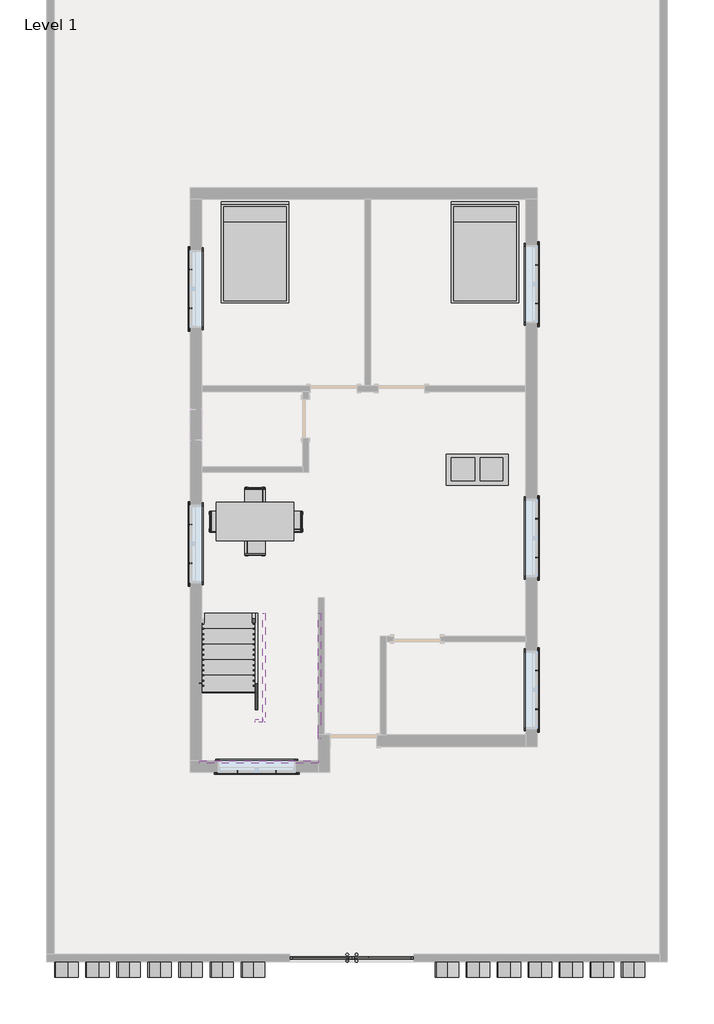
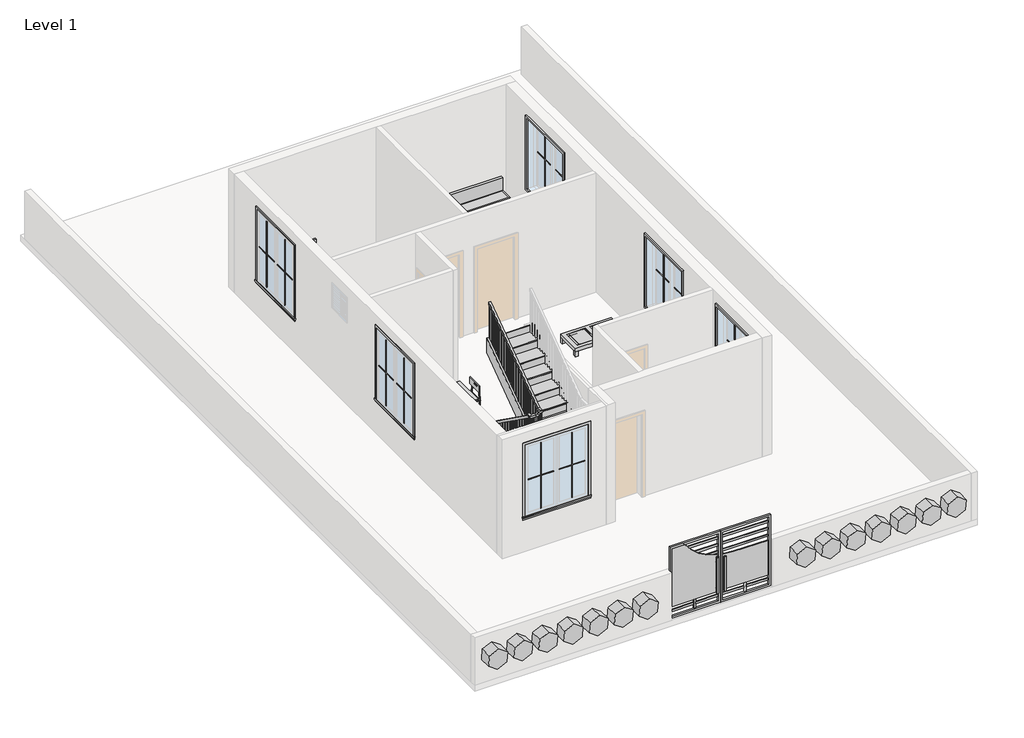
# One storey, part 3 of 3: 40 proxies, 6 members, 3 furniture elements, 1 railing, 1 stair flight.
"""IFC4 building model written with IfcOpenShell, lengths in millimetres."""

from ifc_helpers import new_model, si_unit, frame, origin, place, context, project, spatial, polyline, outline, extrude, faceted_brep, transform, mapped, element, save
from components import generic_models_113f6068, generic_models_1_generic_models_1_1536aad0, generic_models_10_generic_models_1_a884c7fe, generic_models_11_generic_models_1_35dd710a, generic_models_12_generic_models_1_297bb3a6, generic_models_13_generic_models_1_cefb3180, generic_models_14_generic_models_1_e19c2567, generic_models_2_generic_models_1_b64329ca, generic_models_3_generic_models_1_4242ebdf, generic_models_4_generic_models_1_f88cb9c1, generic_models_5_generic_models_1_6c1de215, generic_models_6_generic_models_1_f976f914, generic_models_7_generic_models_1_dc570d8e, generic_models_8_generic_models_1_e8626bb7, generic_models_9_generic_models_1_6881e9d4, muntin_pattern_2x2_muntin_pattern_2x2_f6a80940, muntin_pattern_2x2_muntin_pattern_2x2_09b00a1c, trim_window_exterior_flat_with_sill_698ed857, trim_window_interior_flat_picture_frame_92551a5e, coffee_table_with_brass_mullions_11320_coffee_table_with_5962bef7, bed_17739_bed_17739_15c61121, dining_table_w_chairs_11374_0cdfc61b, stair_flight_d468406d

model = new_model("IFC4")

# Units and contexts
model_context = context("Model", 3, world=origin())
ifc_project = project(units=[si_unit("LENGTHUNIT", "METRE", prefix="MILLI")], contexts=[model_context])

# Site, building, storey
site = spatial("IfcSite", under=ifc_project)
building = spatial("IfcBuilding", under=site)
storey = spatial("IfcBuildingStorey", under=building, Name="Level 1", Elevation=0.0)

# Proxies
placement = place(None, origin())
generic_models_shape = generic_models_113f6068(model_context)
element("IfcBuildingElementProxy", 1, Name="Generic Models", at=placement, inside=storey, context=model_context, shape_type="MappedRepresentation", body=[
    mapped(generic_models_shape, transform((-1286.5514601, -10313.9372434, 0.0), x_axis=(1.0, 0.0, 0.0), y_axis=(0.0, 1.0, 0.0), z_axis=(0.0, 0.0, 1.0))),
])
generic_models_1_generic_models_1_shape = generic_models_1_generic_models_1_1536aad0(model_context)
element("IfcBuildingElementProxy", 2, Name="Generic Models 1 : Generic Models 1", ObjectType="Generic Models 1 : Generic Models 1", at=placement, inside=storey, context=model_context, shape_type="MappedRepresentation", body=[
    mapped(generic_models_1_generic_models_1_shape, transform((0.0, 0.0, 0.0), x_axis=(1.0, 0.0, 0.0), y_axis=(0.0, 1.0, 0.0), z_axis=(0.0, 0.0, 1.0))),
])
generic_models_10_generic_models_1_shape = generic_models_10_generic_models_1_a884c7fe(model_context)
element("IfcBuildingElementProxy", 3, Name="Generic Models 10 : Generic Models 1", ObjectType="Generic Models 10 : Generic Models 1", at=placement, inside=storey, context=model_context, shape_type="MappedRepresentation", body=[
    mapped(generic_models_10_generic_models_1_shape, transform((0.0, 0.0, 0.0), x_axis=(1.0, 0.0, 0.0), y_axis=(0.0, 1.0, 0.0), z_axis=(0.0, 0.0, 1.0))),
])
generic_models_11_generic_models_1_shape = generic_models_11_generic_models_1_35dd710a(model_context)
element("IfcBuildingElementProxy", 4, Name="Generic Models 11 : Generic Models 1", ObjectType="Generic Models 11 : Generic Models 1", at=placement, inside=storey, context=model_context, shape_type="MappedRepresentation", body=[
    mapped(generic_models_11_generic_models_1_shape, transform((0.0, 0.0, 0.0), x_axis=(1.0, 0.0, 0.0), y_axis=(0.0, 1.0, 0.0), z_axis=(0.0, 0.0, 1.0))),
])
generic_models_12_generic_models_1_shape = generic_models_12_generic_models_1_297bb3a6(model_context)
element("IfcBuildingElementProxy", 5, Name="Generic Models 12 : Generic Models 1", ObjectType="Generic Models 12 : Generic Models 1", at=placement, inside=storey, context=model_context, shape_type="MappedRepresentation", body=[
    mapped(generic_models_12_generic_models_1_shape, transform((0.0, 0.0, 0.0), x_axis=(1.0, 0.0, 0.0), y_axis=(0.0, 1.0, 0.0), z_axis=(0.0, 0.0, 1.0))),
])
generic_models_13_generic_models_1_shape = generic_models_13_generic_models_1_cefb3180(model_context)
element("IfcBuildingElementProxy", 6, Name="Generic Models 13 : Generic Models 1", ObjectType="Generic Models 13 : Generic Models 1", at=placement, inside=storey, context=model_context, shape_type="MappedRepresentation", body=[
    mapped(generic_models_13_generic_models_1_shape, transform((0.0, 0.0, 0.0), x_axis=(1.0, 0.0, 0.0), y_axis=(0.0, 1.0, 0.0), z_axis=(0.0, 0.0, 1.0))),
])
generic_models_14_generic_models_1_shape = generic_models_14_generic_models_1_e19c2567(model_context)
element("IfcBuildingElementProxy", 7, Name="Generic Models 14 : Generic Models 1", ObjectType="Generic Models 14 : Generic Models 1", at=placement, inside=storey, context=model_context, shape_type="MappedRepresentation", body=[
    mapped(generic_models_14_generic_models_1_shape, transform((0.0, 0.0, 0.0), x_axis=(1.0, 0.0, 0.0), y_axis=(0.0, 1.0, 0.0), z_axis=(0.0, 0.0, 1.0))),
])
generic_models_2_generic_models_1_shape = generic_models_2_generic_models_1_b64329ca(model_context)
element("IfcBuildingElementProxy", 8, Name="Generic Models 2 : Generic Models 1", ObjectType="Generic Models 2 : Generic Models 1", at=placement, inside=storey, context=model_context, shape_type="MappedRepresentation", body=[
    mapped(generic_models_2_generic_models_1_shape, transform((0.0, 0.0, 0.0), x_axis=(1.0, 0.0, 0.0), y_axis=(0.0, 1.0, 0.0), z_axis=(0.0, 0.0, 1.0))),
])
generic_models_3_generic_models_1_shape = generic_models_3_generic_models_1_4242ebdf(model_context)
element("IfcBuildingElementProxy", 9, Name="Generic Models 3 : Generic Models 1", ObjectType="Generic Models 3 : Generic Models 1", at=placement, inside=storey, context=model_context, shape_type="MappedRepresentation", body=[
    mapped(generic_models_3_generic_models_1_shape, transform((0.0, 0.0, 0.0), x_axis=(1.0, 0.0, 0.0), y_axis=(0.0, 1.0, 0.0), z_axis=(0.0, 0.0, 1.0))),
])
generic_models_4_generic_models_1_shape = generic_models_4_generic_models_1_f88cb9c1(model_context)
element("IfcBuildingElementProxy", 10, Name="Generic Models 4 : Generic Models 1", ObjectType="Generic Models 4 : Generic Models 1", at=placement, inside=storey, context=model_context, shape_type="MappedRepresentation", body=[
    mapped(generic_models_4_generic_models_1_shape, transform((0.0, 0.0, 0.0), x_axis=(1.0, 0.0, 0.0), y_axis=(0.0, 1.0, 0.0), z_axis=(0.0, 0.0, 1.0))),
])
generic_models_5_generic_models_1_shape = generic_models_5_generic_models_1_6c1de215(model_context)
element("IfcBuildingElementProxy", 11, Name="Generic Models 5 : Generic Models 1", ObjectType="Generic Models 5 : Generic Models 1", at=placement, inside=storey, context=model_context, shape_type="MappedRepresentation", body=[
    mapped(generic_models_5_generic_models_1_shape, transform((0.0, 0.0, 0.0), x_axis=(1.0, 0.0, 0.0), y_axis=(0.0, 1.0, 0.0), z_axis=(0.0, 0.0, 1.0))),
])
generic_models_6_generic_models_1_shape = generic_models_6_generic_models_1_f976f914(model_context)
element("IfcBuildingElementProxy", 12, Name="Generic Models 6 : Generic Models 1", ObjectType="Generic Models 6 : Generic Models 1", at=placement, inside=storey, context=model_context, shape_type="MappedRepresentation", body=[
    mapped(generic_models_6_generic_models_1_shape, transform((0.0, 0.0, 0.0), x_axis=(1.0, 0.0, 0.0), y_axis=(0.0, 1.0, 0.0), z_axis=(0.0, 0.0, 1.0))),
])
generic_models_7_generic_models_1_shape = generic_models_7_generic_models_1_dc570d8e(model_context)
element("IfcBuildingElementProxy", 13, Name="Generic Models 7 : Generic Models 1", ObjectType="Generic Models 7 : Generic Models 1", at=placement, inside=storey, context=model_context, shape_type="MappedRepresentation", body=[
    mapped(generic_models_7_generic_models_1_shape, transform((0.0, 0.0, 0.0), x_axis=(1.0, 0.0, 0.0), y_axis=(0.0, 1.0, 0.0), z_axis=(0.0, 0.0, 1.0))),
])
generic_models_8_generic_models_1_shape = generic_models_8_generic_models_1_e8626bb7(model_context)
element("IfcBuildingElementProxy", 14, Name="Generic Models 8 : Generic Models 1", ObjectType="Generic Models 8 : Generic Models 1", at=placement, inside=storey, context=model_context, shape_type="MappedRepresentation", body=[
    mapped(generic_models_8_generic_models_1_shape, transform((0.0, 0.0, 0.0), x_axis=(1.0, 0.0, 0.0), y_axis=(0.0, 1.0, 0.0), z_axis=(0.0, 0.0, 1.0))),
])
generic_models_9_generic_models_1_shape = generic_models_9_generic_models_1_6881e9d4(model_context)
element("IfcBuildingElementProxy", 15, Name="Generic Models 9 : Generic Models 1", ObjectType="Generic Models 9 : Generic Models 1", at=placement, inside=storey, context=model_context, shape_type="MappedRepresentation", body=[
    mapped(generic_models_9_generic_models_1_shape, transform((0.0, 0.0, 0.0), x_axis=(1.0, 0.0, 0.0), y_axis=(0.0, 1.0, 0.0), z_axis=(0.0, 0.0, 1.0))),
])
muntin_pattern_2x2_muntin_pattern_2x2_shape = muntin_pattern_2x2_muntin_pattern_2x2_f6a80940(model_context)
element("IfcBuildingElementProxy", 16, Name="Muntin Pattern_2x2 : Muntin Pattern_2x2", ObjectType="Muntin Pattern_2x2 : Muntin Pattern_2x2", at=placement, inside=storey, context=model_context, shape_type="MappedRepresentation", body=[
    mapped(muntin_pattern_2x2_muntin_pattern_2x2_shape, transform((-2773.368364, -6686.2830018, 984.25), x_axis=(-1.0, 0.0, 0.0), y_axis=(0.0, -1.0, 0.0), z_axis=(0.0, 0.0, 1.0))),
])
element("IfcBuildingElementProxy", 17, Name="Muntin Pattern_2x2 : Muntin Pattern_2x2", ObjectType="Muntin Pattern_2x2 : Muntin Pattern_2x2", at=placement, inside=storey, context=model_context, shape_type="MappedRepresentation", body=[
    mapped(muntin_pattern_2x2_muntin_pattern_2x2_shape, transform((2349.494136, -4693.9705018, 984.25), x_axis=(0.0, -1.0, 0.0), y_axis=(1.0, 0.0, 0.0), z_axis=(0.0, 0.0, 1.0))),
])
element("IfcBuildingElementProxy", 18, Name="Muntin Pattern_2x2 : Muntin Pattern_2x2", ObjectType="Muntin Pattern_2x2 : Muntin Pattern_2x2", at=placement, inside=storey, context=model_context, shape_type="MappedRepresentation", body=[
    mapped(muntin_pattern_2x2_muntin_pattern_2x2_shape, transform((2349.494136, -1712.6455018, 984.25), x_axis=(0.0, -1.0, 0.0), y_axis=(1.0, 0.0, 0.0), z_axis=(0.0, 0.0, 1.0))),
])
element("IfcBuildingElementProxy", 19, Name="Muntin Pattern_2x2 : Muntin Pattern_2x2", ObjectType="Muntin Pattern_2x2 : Muntin Pattern_2x2", at=placement, inside=storey, context=model_context, shape_type="MappedRepresentation", body=[
    mapped(muntin_pattern_2x2_muntin_pattern_2x2_shape, transform((-4451.355864, -2586.5525081, 984.25), x_axis=(0.0, 1.0, 0.0), y_axis=(-1.0, 0.0, 0.0), z_axis=(0.0, 0.0, 1.0))),
])
element("IfcBuildingElementProxy", 20, Name="Muntin Pattern_2x2 : Muntin Pattern_2x2", ObjectType="Muntin Pattern_2x2 : Muntin Pattern_2x2", at=placement, inside=storey, context=model_context, shape_type="MappedRepresentation", body=[
    mapped(muntin_pattern_2x2_muntin_pattern_2x2_shape, transform((2349.494136, 3272.1044982, 984.25), x_axis=(0.0, -1.0, 0.0), y_axis=(1.0, 0.0, 0.0), z_axis=(0.0, 0.0, 1.0))),
])
element("IfcBuildingElementProxy", 21, Name="Muntin Pattern_2x2 : Muntin Pattern_2x2", ObjectType="Muntin Pattern_2x2 : Muntin Pattern_2x2", at=placement, inside=storey, context=model_context, shape_type="MappedRepresentation", body=[
    mapped(muntin_pattern_2x2_muntin_pattern_2x2_shape, transform((-4451.355864, 2421.2162133, 984.25), x_axis=(0.0, 1.0, 0.0), y_axis=(-1.0, 0.0, 0.0), z_axis=(0.0, 0.0, 1.0))),
])
muntin_pattern_2x2_muntin_pattern_2x2_2_shape = muntin_pattern_2x2_muntin_pattern_2x2_09b00a1c(model_context)
element("IfcBuildingElementProxy", 22, Name="Muntin Pattern_2x2 : Muntin Pattern_2x2", ObjectType="Muntin Pattern_2x2 : Muntin Pattern_2x2", at=placement, inside=storey, context=model_context, shape_type="MappedRepresentation", body=[
    mapped(muntin_pattern_2x2_muntin_pattern_2x2_2_shape, transform((-3532.193364, -6686.2830018, 984.25), x_axis=(1.0, 0.0, 0.0), y_axis=(0.0, 1.0, 0.0), z_axis=(0.0, 0.0, 1.0))),
])
element("IfcBuildingElementProxy", 23, Name="Muntin Pattern_2x2 : Muntin Pattern_2x2", ObjectType="Muntin Pattern_2x2 : Muntin Pattern_2x2", at=placement, inside=storey, context=model_context, shape_type="MappedRepresentation", body=[
    mapped(muntin_pattern_2x2_muntin_pattern_2x2_2_shape, transform((2349.494136, -5452.7955018, 984.25), x_axis=(0.0, 1.0, 0.0), y_axis=(-1.0, 0.0, 0.0), z_axis=(0.0, 0.0, 1.0))),
])
element("IfcBuildingElementProxy", 24, Name="Muntin Pattern_2x2 : Muntin Pattern_2x2", ObjectType="Muntin Pattern_2x2 : Muntin Pattern_2x2", at=placement, inside=storey, context=model_context, shape_type="MappedRepresentation", body=[
    mapped(muntin_pattern_2x2_muntin_pattern_2x2_2_shape, transform((2349.494136, -2471.4705018, 984.25), x_axis=(0.0, 1.0, 0.0), y_axis=(-1.0, 0.0, 0.0), z_axis=(0.0, 0.0, 1.0))),
])
element("IfcBuildingElementProxy", 25, Name="Muntin Pattern_2x2 : Muntin Pattern_2x2", ObjectType="Muntin Pattern_2x2 : Muntin Pattern_2x2", at=placement, inside=storey, context=model_context, shape_type="MappedRepresentation", body=[
    mapped(muntin_pattern_2x2_muntin_pattern_2x2_2_shape, transform((-4451.355864, -1827.7275081, 984.25), x_axis=(0.0, -1.0, 0.0), y_axis=(1.0, 0.0, 0.0), z_axis=(0.0, 0.0, 1.0))),
])
element("IfcBuildingElementProxy", 26, Name="Muntin Pattern_2x2 : Muntin Pattern_2x2", ObjectType="Muntin Pattern_2x2 : Muntin Pattern_2x2", at=placement, inside=storey, context=model_context, shape_type="MappedRepresentation", body=[
    mapped(muntin_pattern_2x2_muntin_pattern_2x2_2_shape, transform((2349.494136, 2513.2794982, 984.25), x_axis=(0.0, 1.0, 0.0), y_axis=(-1.0, 0.0, 0.0), z_axis=(0.0, 0.0, 1.0))),
])
element("IfcBuildingElementProxy", 27, Name="Muntin Pattern_2x2 : Muntin Pattern_2x2", ObjectType="Muntin Pattern_2x2 : Muntin Pattern_2x2", at=placement, inside=storey, context=model_context, shape_type="MappedRepresentation", body=[
    mapped(muntin_pattern_2x2_muntin_pattern_2x2_2_shape, transform((-4451.355864, 3180.0412133, 984.25), x_axis=(0.0, -1.0, 0.0), y_axis=(1.0, 0.0, 0.0), z_axis=(0.0, 0.0, 1.0))),
])
trim_window_exterior_flat_with_sill_shape = trim_window_exterior_flat_with_sill_698ed857(model_context)
element("IfcBuildingElementProxy", 28, Name="Trim-Window-Exterior-Flat : with Sill", ObjectType="Trim-Window-Exterior-Flat : with Sill", at=placement, inside=storey, context=model_context, shape_type="MappedRepresentation", body=[
    mapped(trim_window_exterior_flat_with_sill_shape, transform((-3152.780864, -6695.8080018, 2743.2), x_axis=(1.0, 0.0, 0.0), y_axis=(0.0, 0.0, 1.0), z_axis=(0.0, -1.0, 0.0))),
])
element("IfcBuildingElementProxy", 29, Name="Trim-Window-Exterior-Flat : with Sill", ObjectType="Trim-Window-Exterior-Flat : with Sill", at=placement, inside=storey, context=model_context, shape_type="MappedRepresentation", body=[
    mapped(trim_window_exterior_flat_with_sill_shape, transform((2359.019136, -5073.3830018, 2743.2), x_axis=(0.0, 1.0, 0.0), y_axis=(0.0, 0.0, 1.0), z_axis=(1.0, 0.0, 0.0))),
])
element("IfcBuildingElementProxy", 30, Name="Trim-Window-Exterior-Flat : with Sill", ObjectType="Trim-Window-Exterior-Flat : with Sill", at=placement, inside=storey, context=model_context, shape_type="MappedRepresentation", body=[
    mapped(trim_window_exterior_flat_with_sill_shape, transform((2359.019136, -2092.0580018, 2743.2), x_axis=(0.0, 1.0, 0.0), y_axis=(0.0, 0.0, 1.0), z_axis=(1.0, 0.0, 0.0))),
])
element("IfcBuildingElementProxy", 31, Name="Trim-Window-Exterior-Flat : with Sill", ObjectType="Trim-Window-Exterior-Flat : with Sill", at=placement, inside=storey, context=model_context, shape_type="MappedRepresentation", body=[
    mapped(trim_window_exterior_flat_with_sill_shape, transform((-4460.880864, -2207.1400081, 2743.2), x_axis=(0.0, -1.0, 0.0), y_axis=(0.0, 0.0, 1.0), z_axis=(-1.0, 0.0, 0.0))),
])
element("IfcBuildingElementProxy", 32, Name="Trim-Window-Exterior-Flat : with Sill", ObjectType="Trim-Window-Exterior-Flat : with Sill", at=placement, inside=storey, context=model_context, shape_type="MappedRepresentation", body=[
    mapped(trim_window_exterior_flat_with_sill_shape, transform((2359.019136, 2892.6919982, 2743.2), x_axis=(0.0, 1.0, 0.0), y_axis=(0.0, 0.0, 1.0), z_axis=(1.0, 0.0, 0.0))),
])
element("IfcBuildingElementProxy", 33, Name="Trim-Window-Exterior-Flat : with Sill", ObjectType="Trim-Window-Exterior-Flat : with Sill", at=placement, inside=storey, context=model_context, shape_type="MappedRepresentation", body=[
    mapped(trim_window_exterior_flat_with_sill_shape, transform((-4460.880864, 2800.6287133, 2743.2), x_axis=(0.0, -1.0, 0.0), y_axis=(0.0, 0.0, 1.0), z_axis=(-1.0, 0.0, 0.0))),
])
trim_window_interior_flat_picture_frame_shape = trim_window_interior_flat_picture_frame_92551a5e(model_context)
element("IfcBuildingElementProxy", 34, Name="Trim-Window-Interior-Flat : Picture Frame", ObjectType="Trim-Window-Interior-Flat : Picture Frame", at=placement, inside=storey, context=model_context, shape_type="MappedRepresentation", body=[
    mapped(trim_window_interior_flat_picture_frame_shape, transform((-3152.780864, -6467.2080018, 2743.2), x_axis=(-1.0, 0.0, 0.0), y_axis=(0.0, 0.0, 1.0), z_axis=(0.0, 1.0, 0.0))),
])
element("IfcBuildingElementProxy", 35, Name="Trim-Window-Interior-Flat : Picture Frame", ObjectType="Trim-Window-Interior-Flat : Picture Frame", at=placement, inside=storey, context=model_context, shape_type="MappedRepresentation", body=[
    mapped(trim_window_interior_flat_picture_frame_shape, transform((2130.419136, -5073.3830018, 2743.2), x_axis=(0.0, -1.0, 0.0), y_axis=(0.0, 0.0, 1.0), z_axis=(-1.0, 0.0, 0.0))),
])
element("IfcBuildingElementProxy", 36, Name="Trim-Window-Interior-Flat : Picture Frame", ObjectType="Trim-Window-Interior-Flat : Picture Frame", at=placement, inside=storey, context=model_context, shape_type="MappedRepresentation", body=[
    mapped(trim_window_interior_flat_picture_frame_shape, transform((2130.419136, -2092.0580018, 2743.2), x_axis=(0.0, -1.0, 0.0), y_axis=(0.0, 0.0, 1.0), z_axis=(-1.0, 0.0, 0.0))),
])
element("IfcBuildingElementProxy", 37, Name="Trim-Window-Interior-Flat : Picture Frame", ObjectType="Trim-Window-Interior-Flat : Picture Frame", at=placement, inside=storey, context=model_context, shape_type="MappedRepresentation", body=[
    mapped(trim_window_interior_flat_picture_frame_shape, transform((-4232.280864, -2207.1400081, 2743.2), x_axis=(0.0, 1.0, 0.0), y_axis=(0.0, 0.0, 1.0), z_axis=(1.0, 0.0, 0.0))),
])
element("IfcBuildingElementProxy", 38, Name="Trim-Window-Interior-Flat : Picture Frame", ObjectType="Trim-Window-Interior-Flat : Picture Frame", at=placement, inside=storey, context=model_context, shape_type="MappedRepresentation", body=[
    mapped(trim_window_interior_flat_picture_frame_shape, transform((2130.419136, 2892.6919982, 2743.2), x_axis=(0.0, -1.0, 0.0), y_axis=(0.0, 0.0, 1.0), z_axis=(-1.0, 0.0, 0.0))),
])
element("IfcBuildingElementProxy", 39, Name="Trim-Window-Interior-Flat : Picture Frame", ObjectType="Trim-Window-Interior-Flat : Picture Frame", at=placement, inside=storey, context=model_context, shape_type="MappedRepresentation", body=[
    mapped(trim_window_interior_flat_picture_frame_shape, transform((-4232.280864, 2800.6287133, 2743.2), x_axis=(0.0, 1.0, 0.0), y_axis=(0.0, 0.0, 1.0), z_axis=(1.0, 0.0, 0.0))),
])
coffee_table_with_brass_mullions_11320_coffee_table_with_shape = coffee_table_with_brass_mullions_11320_coffee_table_with_5962bef7(model_context)
element("IfcBuildingElementProxy", 40, Name="coffee_table_with_brass_mullions_11320 : coffee_table_with_brass_mullions_11320", ObjectType="coffee_table_with_brass_mullions_11320 : coffee_table_with_brass_mullions_11320", at=placement, inside=storey, context=model_context, shape_type="MappedRepresentation", body=[
    mapped(coffee_table_with_brass_mullions_11320_coffee_table_with_shape, transform((1812.3816081, -1181.1001099, 0.0), x_axis=(1.0, 0.0, 0.0), y_axis=(0.0, 1.0, 0.0), z_axis=(0.0, 0.0, 1.0))),
])

# Furniture
bed_17739_bed_17739_shape = bed_17739_bed_17739_15c61121(model_context)
element("IfcFurniture", 41, ObjectType="Bed_17739 : Bed_17739", at=placement, inside=storey, context=model_context, shape_type="MappedRepresentation", body=[
    mapped(bed_17739_bed_17739_shape, transform((1328.5116081, 3496.3098901, 0.0), x_axis=(1.0, 0.0, 0.0), y_axis=(0.0, 1.0, 0.0), z_axis=(0.0, 0.0, 1.0))),
])
element("IfcFurniture", 42, ObjectType="Bed_17739 : Bed_17739", at=placement, inside=storey, context=model_context, shape_type="MappedRepresentation", body=[
    mapped(bed_17739_bed_17739_shape, transform((-3187.6083919, 3496.3098901, 0.0), x_axis=(1.0, 0.0, 0.0), y_axis=(0.0, 1.0, 0.0), z_axis=(0.0, 0.0, 1.0))),
])
dining_table_w_chairs_11374_shape = dining_table_w_chairs_11374_0cdfc61b(model_context)
element("IfcFurniture", 43, ObjectType="Dining_Table_w_Chairs_11374", at=placement, inside=storey, context=model_context, shape_type="MappedRepresentation", body=[
    mapped(dining_table_w_chairs_11374_shape, transform((-3205.8741586, -1863.0511877, 0.0), x_axis=(1.0, 0.0, 0.0), y_axis=(0.0, 1.0, 0.0), z_axis=(0.0, 0.0, 1.0))),
])

# Members
element("IfcMember", 44, ObjectType="Stringer - 2\" Width", at=placement, inside=storey, context=model_context, shape_type="SweptSolid", body=[
    extrude(outline(polyline([(-3571.6080018, 223.0558696), (-3571.6080018, 0.0), (-3783.7275327, 0.0), (-5654.4080018, 1336.2003351), (-5654.4080018, 1710.7701553), (-3571.6080018, 223.0558696)])), frame((-3187.6083919, 0.0, 0.0), z_axis=(1.0, 0.0, 0.0), x_axis=(0.0, 1.0, 0.0)), (0.0, 0.0, 1.0), 50.8),
])
element("IfcMember", 45, ObjectType="Stringer - 2\" Width", at=placement, inside=storey, context=model_context, shape_type="SweptSolid", body=[
    extrude(outline(polyline([(-3187.6083919, -5705.2080018), (-3187.6083919, -5654.4080018), (-3035.2083919, -5654.4080018), (-3035.2083919, -5705.2080018), (-3187.6083919, -5705.2080018)])), frame((0.0, 0.0, 1513.1142857), z_axis=(0.0, 0.0, 1.0), x_axis=(1.0, 0.0, 0.0)), (0.0, 0.0, 1.0), 304.8),
])
element("IfcMember", 46, ObjectType="Stringer - 2\" Width", at=placement, inside=storey, context=model_context, shape_type="SweptSolid", body=[
    extrude(outline(polyline([(-5705.2080018, 1513.1142857), (-5705.2080018, 1747.0558696), (-3571.6080018, 3271.0558696), (-3571.6080018, 2896.4860494), (-5508.3284709, 1513.1142857), (-5705.2080018, 1513.1142857)])), frame((-3035.2083919, 0.0, 0.0), z_axis=(1.0, 0.0, 0.0), x_axis=(0.0, 1.0, 0.0)), (0.0, 0.0, 1.0), 50.8),
])
element("IfcMember", 47, ObjectType="Stringer - 2\" Width", at=placement, inside=storey, context=model_context, shape_type="SweptSolid", body=[
    extrude(outline(polyline([(-3571.6080018, 223.0558696), (-3571.6080018, 0.0), (-3783.7275327, 0.0), (-6328.8075327, 1817.9142857), (-5804.4097844, 1817.9142857), (-3571.6080018, 223.0558696)])), frame((-4283.080864, 0.0, 0.0), z_axis=(1.0, 0.0, 0.0), x_axis=(0.0, 1.0, 0.0)), (0.0, 0.0, 1.0), 50.8),
])
element("IfcMember", 48, ObjectType="Stringer - 2\" Width", at=placement, inside=storey, context=model_context, shape_type="SweptSolid", body=[
    extrude(outline(polyline([(-4283.080864, -6518.0080018), (-4283.080864, -6467.2080018), (-1946.280864, -6467.2080018), (-1946.280864, -6518.0080018), (-4283.080864, -6518.0080018)])), frame((0.0, 0.0, 1513.1142857), z_axis=(0.0, 0.0, 1.0), x_axis=(1.0, 0.0, 0.0)), (0.0, 0.0, 1.0), 304.8),
])
element("IfcMember", 49, ObjectType="Stringer - 2\" Width", at=placement, inside=storey, context=model_context, shape_type="SweptSolid", body=[
    extrude(outline(polyline([(-6032.7262192, 1513.1142857), (-3571.6080018, 3271.0558696), (-3571.6080018, 2896.4860494), (-5508.3284709, 1513.1142857), (-6032.7262192, 1513.1142857)])), frame((-1946.280864, 0.0, 0.0), z_axis=(1.0, 0.0, 0.0), x_axis=(0.0, 1.0, 0.0)), (0.0, 0.0, 1.0), 50.8),
])

# Railing
element("IfcRailing", 50, ObjectType="Handrail - Rectangular", at=placement, inside=storey, context=model_context, shape_type="SolidModel", body=[
    faceted_brep([(-3187.6083919, -3571.6080018, 1132.1142857), (-3187.6083919, -3571.6080018, 1069.6859823), (-3238.4083919, -3571.6080018, 1069.6859823), (-3238.4083919, -3571.6080018, 1132.1142857), (-3187.6083919, -5629.0080018, 2601.6857143), (-3187.6083919, -5679.8080018, 2575.5431252), (-3238.4083919, -5679.8080018, 2575.5431252), (-3238.4083919, -5629.0080018, 2601.6857143), (-3187.6083919, -5629.0080018, 2656.1142857), (-3187.6083919, -5679.8080018, 2605.3142857), (-3238.4083919, -5679.8080018, 2605.3142857), (-3238.4083919, -5629.0080018, 2656.1142857), (-3187.6083919, -5705.2080018, 2656.1142857), (-3187.6083919, -5705.2080018, 2605.3142857), (-3238.4083919, -5756.0080018, 2605.3142857), (-3238.4083919, -5756.0080018, 2656.1142857), (-3111.4083919, -5705.2080018, 2656.1142857), (-3111.4083919, -5705.2080018, 2605.3142857), (-3111.4083919, -5756.0080018, 2605.3142857), (-3111.4083919, -5756.0080018, 2656.1142857), (-3060.6083919, -5705.2080018, 2656.1142857), (-3009.8083919, -5705.2080018, 2605.3142857), (-3009.8083919, -5756.0080018, 2605.3142857), (-3060.6083919, -5756.0080018, 2656.1142857), (-3060.6083919, -5705.2080018, 2710.5428571), (-3009.8083919, -5705.2080018, 2659.7428571), (-3009.8083919, -5756.0080018, 2659.7428571), (-3060.6083919, -5756.0080018, 2710.5428571), (-2984.4083919, -5705.2080018, 2710.5428571), (-2984.4083919, -5705.2080018, 2659.7428571), (-2933.6083919, -5756.0080018, 2659.7428571), (-2933.6083919, -5756.0080018, 2710.5428571), (-2984.4083919, -5629.0080018, 2710.5428571), (-2984.4083919, -5612.7283771, 2659.7428571), (-2933.6083919, -5612.7283771, 2659.7428571), (-2933.6083919, -5629.0080018, 2710.5428571), (-2984.4083919, -3571.6080018, 4180.1142857), (-2933.6083919, -3571.6080018, 4180.1142857), (-2933.6083919, -3571.6080018, 4117.6859823), (-2984.4083919, -3571.6080018, 4117.6859823)], [[[0, 1, 2, 3]], [[1, 0, 4, 5]], [[2, 1, 5, 6]], [[3, 2, 6, 7]], [[0, 3, 7, 4]], [[5, 4, 8, 9]], [[6, 5, 9, 10]], [[7, 6, 10, 11]], [[4, 7, 11, 8]], [[9, 8, 12, 13]], [[10, 9, 13, 14]], [[11, 10, 14, 15]], [[8, 11, 15, 12]], [[13, 12, 16, 17]], [[14, 13, 17, 18]], [[15, 14, 18, 19]], [[12, 15, 19, 16]], [[17, 16, 20, 21]], [[18, 17, 21, 22]], [[19, 18, 22, 23]], [[16, 19, 23, 20]], [[21, 20, 24, 25]], [[22, 21, 25, 26]], [[23, 22, 26, 27]], [[20, 23, 27, 24]], [[25, 24, 28, 29]], [[26, 25, 29, 30]], [[27, 26, 30, 31]], [[24, 27, 31, 28]], [[29, 28, 32, 33]], [[30, 29, 33, 34]], [[31, 30, 34, 35]], [[28, 31, 35, 32]], [[36, 37, 38, 39]], [[33, 32, 36, 39]], [[34, 33, 39, 38]], [[35, 34, 38, 37]], [[32, 35, 37, 36]]]),
    extrude(outline(polyline([(-3587.4830018, 4106.3466966), (-3587.4830018, 3048.0), (-3606.5330018, 3048.0), (-3606.5330018, 4092.7395538), (-3587.4830018, 4106.3466966)])), frame((-2968.5333919, 0.0, 0.0), z_axis=(1.0, 0.0, 0.0), x_axis=(0.0, 1.0, 0.0)), (0.0, 0.0, 1.0), 19.05),
    extrude(outline(polyline([(-3689.0830018, 4033.7752681), (-3689.0830018, 3048.0), (-3708.1330018, 3048.0), (-3708.1330018, 4020.1681252), (-3689.0830018, 4033.7752681)])), frame((-2968.5333919, 0.0, 0.0), z_axis=(1.0, 0.0, 0.0), x_axis=(0.0, 1.0, 0.0)), (0.0, 0.0, 1.0), 19.05),
    extrude(outline(polyline([(-3790.6830018, 3961.2038395), (-3790.6830018, 3048.0), (-3809.7330018, 3048.0), (-3809.7330018, 3947.5966966), (-3790.6830018, 3961.2038395)])), frame((-2968.5333919, 0.0, 0.0), z_axis=(1.0, 0.0, 0.0), x_axis=(0.0, 1.0, 0.0)), (0.0, 0.0, 1.0), 19.05),
    extrude(outline(polyline([(-3892.2830018, 3888.6324109), (-3892.2830018, 2830.2857143), (-3911.3330018, 2830.2857143), (-3911.3330018, 3875.0252681), (-3892.2830018, 3888.6324109)])), frame((-2968.5333919, 0.0, 0.0), z_axis=(1.0, 0.0, 0.0), x_axis=(0.0, 1.0, 0.0)), (0.0, 0.0, 1.0), 19.05),
    extrude(outline(polyline([(-3993.8830018, 3816.0609823), (-3993.8830018, 2830.2857143), (-4012.9330018, 2830.2857143), (-4012.9330018, 3802.4538395), (-3993.8830018, 3816.0609823)])), frame((-2968.5333919, 0.0, 0.0), z_axis=(1.0, 0.0, 0.0), x_axis=(0.0, 1.0, 0.0)), (0.0, 0.0, 1.0), 19.05),
    extrude(outline(polyline([(-4095.4830018, 3743.4895538), (-4095.4830018, 2830.2857143), (-4114.5330018, 2830.2857143), (-4114.5330018, 3729.8824109), (-4095.4830018, 3743.4895538)])), frame((-2968.5333919, 0.0, 0.0), z_axis=(1.0, 0.0, 0.0), x_axis=(0.0, 1.0, 0.0)), (0.0, 0.0, 1.0), 19.05),
    extrude(outline(polyline([(-4197.0830018, 3670.9181252), (-4197.0830018, 2612.5714286), (-4216.1330018, 2612.5714286), (-4216.1330018, 3657.3109823), (-4197.0830018, 3670.9181252)])), frame((-2968.5333919, 0.0, 0.0), z_axis=(1.0, 0.0, 0.0), x_axis=(0.0, 1.0, 0.0)), (0.0, 0.0, 1.0), 19.05),
    extrude(outline(polyline([(-4298.6830018, 3598.3466966), (-4298.6830018, 2612.5714286), (-4317.7330018, 2612.5714286), (-4317.7330018, 3584.7395538), (-4298.6830018, 3598.3466966)])), frame((-2968.5333919, 0.0, 0.0), z_axis=(1.0, 0.0, 0.0), x_axis=(0.0, 1.0, 0.0)), (0.0, 0.0, 1.0), 19.05),
    extrude(outline(polyline([(-4400.2830018, 3525.7752681), (-4400.2830018, 2612.5714286), (-4419.3330018, 2612.5714286), (-4419.3330018, 3512.1681252), (-4400.2830018, 3525.7752681)])), frame((-2968.5333919, 0.0, 0.0), z_axis=(1.0, 0.0, 0.0), x_axis=(0.0, 1.0, 0.0)), (0.0, 0.0, 1.0), 19.05),
    extrude(outline(polyline([(-4501.8830018, 3453.2038395), (-4501.8830018, 2394.8571429), (-4520.9330018, 2394.8571429), (-4520.9330018, 3439.5966966), (-4501.8830018, 3453.2038395)])), frame((-2968.5333919, 0.0, 0.0), z_axis=(1.0, 0.0, 0.0), x_axis=(0.0, 1.0, 0.0)), (0.0, 0.0, 1.0), 19.05),
    extrude(outline(polyline([(-4603.4830018, 3380.6324109), (-4603.4830018, 2394.8571429), (-4622.5330018, 2394.8571429), (-4622.5330018, 3367.0252681), (-4603.4830018, 3380.6324109)])), frame((-2968.5333919, 0.0, 0.0), z_axis=(1.0, 0.0, 0.0), x_axis=(0.0, 1.0, 0.0)), (0.0, 0.0, 1.0), 19.05),
    extrude(outline(polyline([(-4705.0830018, 3308.0609823), (-4705.0830018, 2394.8571429), (-4724.1330018, 2394.8571429), (-4724.1330018, 3294.4538395), (-4705.0830018, 3308.0609823)])), frame((-2968.5333919, 0.0, 0.0), z_axis=(1.0, 0.0, 0.0), x_axis=(0.0, 1.0, 0.0)), (0.0, 0.0, 1.0), 19.05),
    extrude(outline(polyline([(-4806.6830018, 3235.4895538), (-4806.6830018, 2177.1428571), (-4825.7330018, 2177.1428571), (-4825.7330018, 3221.8824109), (-4806.6830018, 3235.4895538)])), frame((-2968.5333919, 0.0, 0.0), z_axis=(1.0, 0.0, 0.0), x_axis=(0.0, 1.0, 0.0)), (0.0, 0.0, 1.0), 19.05),
    extrude(outline(polyline([(-4908.2830018, 3162.9181252), (-4908.2830018, 2177.1428571), (-4927.3330018, 2177.1428571), (-4927.3330018, 3149.3109823), (-4908.2830018, 3162.9181252)])), frame((-2968.5333919, 0.0, 0.0), z_axis=(1.0, 0.0, 0.0), x_axis=(0.0, 1.0, 0.0)), (0.0, 0.0, 1.0), 19.05),
    extrude(outline(polyline([(-5009.8830018, 3090.3466966), (-5009.8830018, 2177.1428571), (-5028.9330018, 2177.1428571), (-5028.9330018, 3076.7395538), (-5009.8830018, 3090.3466966)])), frame((-2968.5333919, 0.0, 0.0), z_axis=(1.0, 0.0, 0.0), x_axis=(0.0, 1.0, 0.0)), (0.0, 0.0, 1.0), 19.05),
    extrude(outline(polyline([(-5111.4830018, 3017.7752681), (-5111.4830018, 1959.4285714), (-5130.5330018, 1959.4285714), (-5130.5330018, 3004.1681252), (-5111.4830018, 3017.7752681)])), frame((-2968.5333919, 0.0, 0.0), z_axis=(1.0, 0.0, 0.0), x_axis=(0.0, 1.0, 0.0)), (0.0, 0.0, 1.0), 19.05),
    extrude(outline(polyline([(-5213.0830018, 2945.2038395), (-5213.0830018, 1959.4285714), (-5232.1330018, 1959.4285714), (-5232.1330018, 2931.5966966), (-5213.0830018, 2945.2038395)])), frame((-2968.5333919, 0.0, 0.0), z_axis=(1.0, 0.0, 0.0), x_axis=(0.0, 1.0, 0.0)), (0.0, 0.0, 1.0), 19.05),
    extrude(outline(polyline([(-5314.6830018, 2872.6324109), (-5314.6830018, 1959.4285714), (-5333.7330018, 1959.4285714), (-5333.7330018, 2859.0252681), (-5314.6830018, 2872.6324109)])), frame((-2968.5333919, 0.0, 0.0), z_axis=(1.0, 0.0, 0.0), x_axis=(0.0, 1.0, 0.0)), (0.0, 0.0, 1.0), 19.05),
    extrude(outline(polyline([(-5416.2830018, 2800.0609823), (-5416.2830018, 1741.7142857), (-5435.3330018, 1741.7142857), (-5435.3330018, 2786.4538395), (-5416.2830018, 2800.0609823)])), frame((-2968.5333919, 0.0, 0.0), z_axis=(1.0, 0.0, 0.0), x_axis=(0.0, 1.0, 0.0)), (0.0, 0.0, 1.0), 19.05),
    extrude(outline(polyline([(-5517.8830018, 2727.4895538), (-5517.8830018, 1741.7142857), (-5536.9330018, 1741.7142857), (-5536.9330018, 2713.8824109), (-5517.8830018, 2727.4895538)])), frame((-2968.5333919, 0.0, 0.0), z_axis=(1.0, 0.0, 0.0), x_axis=(0.0, 1.0, 0.0)), (0.0, 0.0, 1.0), 19.05),
    extrude(outline(polyline([(-5619.4830018, 2654.9181252), (-5619.4830018, 1741.7142857), (-5638.5330018, 1741.7142857), (-5638.5330018, 2641.3109823), (-5619.4830018, 2654.9181252)])), frame((-2968.5333919, 0.0, 0.0), z_axis=(1.0, 0.0, 0.0), x_axis=(0.0, 1.0, 0.0)), (0.0, 0.0, 1.0), 19.05),
    extrude(outline(polyline([(-3019.3333919, -5721.0830018), (-3000.2833919, -5721.0830018), (-3000.2833919, -5740.1330018), (-3019.3333919, -5740.1330018), (-3019.3333919, -5721.0830018)])), frame((0.0, 0.0, 1741.7142857), z_axis=(0.0, 0.0, 1.0), x_axis=(1.0, 0.0, 0.0)), (0.0, 0.0, 1.0), 918.0285714),
    extrude(outline(polyline([(-3120.9333919, -5721.0830018), (-3101.8833919, -5721.0830018), (-3101.8833919, -5740.1330018), (-3120.9333919, -5740.1330018), (-3120.9333919, -5721.0830018)])), frame((0.0, 0.0, 1741.7142857), z_axis=(0.0, 0.0, 1.0), x_axis=(1.0, 0.0, 0.0)), (0.0, 0.0, 1.0), 863.6),
    extrude(outline(polyline([(-3203.4833919, -5695.6830018), (-3203.4833919, -5714.7330018), (-3222.5333919, -5714.7330018), (-3222.5333919, -5695.6830018), (-3203.4833919, -5695.6830018)])), frame((0.0, 0.0, 1741.7142857), z_axis=(0.0, 0.0, 1.0), x_axis=(1.0, 0.0, 0.0)), (0.0, 0.0, 1.0), 863.6),
    extrude(outline(polyline([(-5594.0830018, 2514.3109823), (-5594.0830018, 1524.0), (-5613.1330018, 1524.0), (-5613.1330018, 2527.9181252), (-5594.0830018, 2514.3109823)])), frame((-3222.5333919, 0.0, 0.0), z_axis=(1.0, 0.0, 0.0), x_axis=(0.0, 1.0, 0.0)), (0.0, 0.0, 1.0), 19.05),
    extrude(outline(polyline([(-5492.4830018, 2441.7395538), (-5492.4830018, 1524.0), (-5511.5330018, 1524.0), (-5511.5330018, 2455.3466966), (-5492.4830018, 2441.7395538)])), frame((-3222.5333919, 0.0, 0.0), z_axis=(1.0, 0.0, 0.0), x_axis=(0.0, 1.0, 0.0)), (0.0, 0.0, 1.0), 19.05),
    extrude(outline(polyline([(-5390.8830018, 2369.1681252), (-5390.8830018, 1524.0), (-5409.9330018, 1524.0), (-5409.9330018, 2382.7752681), (-5390.8830018, 2369.1681252)])), frame((-3222.5333919, 0.0, 0.0), z_axis=(1.0, 0.0, 0.0), x_axis=(0.0, 1.0, 0.0)), (0.0, 0.0, 1.0), 19.05),
    extrude(outline(polyline([(-5289.2830018, 2296.5966966), (-5289.2830018, 1306.2857143), (-5308.3330018, 1306.2857143), (-5308.3330018, 2310.2038395), (-5289.2830018, 2296.5966966)])), frame((-3222.5333919, 0.0, 0.0), z_axis=(1.0, 0.0, 0.0), x_axis=(0.0, 1.0, 0.0)), (0.0, 0.0, 1.0), 19.05),
    extrude(outline(polyline([(-5187.6830018, 2224.0252681), (-5187.6830018, 1306.2857143), (-5206.7330018, 1306.2857143), (-5206.7330018, 2237.6324109), (-5187.6830018, 2224.0252681)])), frame((-3222.5333919, 0.0, 0.0), z_axis=(1.0, 0.0, 0.0), x_axis=(0.0, 1.0, 0.0)), (0.0, 0.0, 1.0), 19.05),
    extrude(outline(polyline([(-5086.0830018, 2151.4538395), (-5086.0830018, 1306.2857143), (-5105.1330018, 1306.2857143), (-5105.1330018, 2165.0609823), (-5086.0830018, 2151.4538395)])), frame((-3222.5333919, 0.0, 0.0), z_axis=(1.0, 0.0, 0.0), x_axis=(0.0, 1.0, 0.0)), (0.0, 0.0, 1.0), 19.05),
    extrude(outline(polyline([(-4984.4830018, 2078.8824109), (-4984.4830018, 1088.5714286), (-5003.5330018, 1088.5714286), (-5003.5330018, 2092.4895538), (-4984.4830018, 2078.8824109)])), frame((-3222.5333919, 0.0, 0.0), z_axis=(1.0, 0.0, 0.0), x_axis=(0.0, 1.0, 0.0)), (0.0, 0.0, 1.0), 19.05),
    extrude(outline(polyline([(-4882.8830018, 2006.3109823), (-4882.8830018, 1088.5714286), (-4901.9330018, 1088.5714286), (-4901.9330018, 2019.9181252), (-4882.8830018, 2006.3109823)])), frame((-3222.5333919, 0.0, 0.0), z_axis=(1.0, 0.0, 0.0), x_axis=(0.0, 1.0, 0.0)), (0.0, 0.0, 1.0), 19.05),
    extrude(outline(polyline([(-4781.2830018, 1933.7395538), (-4781.2830018, 1088.5714286), (-4800.3330018, 1088.5714286), (-4800.3330018, 1947.3466966), (-4781.2830018, 1933.7395538)])), frame((-3222.5333919, 0.0, 0.0), z_axis=(1.0, 0.0, 0.0), x_axis=(0.0, 1.0, 0.0)), (0.0, 0.0, 1.0), 19.05),
    extrude(outline(polyline([(-4679.6830018, 1861.1681252), (-4679.6830018, 870.8571429), (-4698.7330018, 870.8571429), (-4698.7330018, 1874.7752681), (-4679.6830018, 1861.1681252)])), frame((-3222.5333919, 0.0, 0.0), z_axis=(1.0, 0.0, 0.0), x_axis=(0.0, 1.0, 0.0)), (0.0, 0.0, 1.0), 19.05),
    extrude(outline(polyline([(-4578.0830018, 1788.5966966), (-4578.0830018, 870.8571429), (-4597.1330018, 870.8571429), (-4597.1330018, 1802.2038395), (-4578.0830018, 1788.5966966)])), frame((-3222.5333919, 0.0, 0.0), z_axis=(1.0, 0.0, 0.0), x_axis=(0.0, 1.0, 0.0)), (0.0, 0.0, 1.0), 19.05),
    extrude(outline(polyline([(-4476.4830018, 1716.0252681), (-4476.4830018, 870.8571429), (-4495.5330018, 870.8571429), (-4495.5330018, 1729.6324109), (-4476.4830018, 1716.0252681)])), frame((-3222.5333919, 0.0, 0.0), z_axis=(1.0, 0.0, 0.0), x_axis=(0.0, 1.0, 0.0)), (0.0, 0.0, 1.0), 19.05),
    extrude(outline(polyline([(-4374.8830018, 1643.4538395), (-4374.8830018, 653.1428571), (-4393.9330018, 653.1428571), (-4393.9330018, 1657.0609823), (-4374.8830018, 1643.4538395)])), frame((-3222.5333919, 0.0, 0.0), z_axis=(1.0, 0.0, 0.0), x_axis=(0.0, 1.0, 0.0)), (0.0, 0.0, 1.0), 19.05),
    extrude(outline(polyline([(-4273.2830018, 1570.8824109), (-4273.2830018, 653.1428571), (-4292.3330018, 653.1428571), (-4292.3330018, 1584.4895538), (-4273.2830018, 1570.8824109)])), frame((-3222.5333919, 0.0, 0.0), z_axis=(1.0, 0.0, 0.0), x_axis=(0.0, 1.0, 0.0)), (0.0, 0.0, 1.0), 19.05),
    extrude(outline(polyline([(-4171.6830018, 1498.3109823), (-4171.6830018, 653.1428571), (-4190.7330018, 653.1428571), (-4190.7330018, 1511.9181252), (-4171.6830018, 1498.3109823)])), frame((-3222.5333919, 0.0, 0.0), z_axis=(1.0, 0.0, 0.0), x_axis=(0.0, 1.0, 0.0)), (0.0, 0.0, 1.0), 19.05),
    extrude(outline(polyline([(-4070.0830018, 1425.7395538), (-4070.0830018, 435.4285714), (-4089.1330018, 435.4285714), (-4089.1330018, 1439.3466966), (-4070.0830018, 1425.7395538)])), frame((-3222.5333919, 0.0, 0.0), z_axis=(1.0, 0.0, 0.0), x_axis=(0.0, 1.0, 0.0)), (0.0, 0.0, 1.0), 19.05),
    extrude(outline(polyline([(-3968.4830018, 1353.1681252), (-3968.4830018, 435.4285714), (-3987.5330018, 435.4285714), (-3987.5330018, 1366.7752681), (-3968.4830018, 1353.1681252)])), frame((-3222.5333919, 0.0, 0.0), z_axis=(1.0, 0.0, 0.0), x_axis=(0.0, 1.0, 0.0)), (0.0, 0.0, 1.0), 19.05),
    extrude(outline(polyline([(-3866.8830018, 1280.5966966), (-3866.8830018, 435.4285714), (-3885.9330018, 435.4285714), (-3885.9330018, 1294.2038395), (-3866.8830018, 1280.5966966)])), frame((-3222.5333919, 0.0, 0.0), z_axis=(1.0, 0.0, 0.0), x_axis=(0.0, 1.0, 0.0)), (0.0, 0.0, 1.0), 19.05),
    extrude(outline(polyline([(-3765.2830018, 1208.0252681), (-3765.2830018, 217.7142857), (-3784.3330018, 217.7142857), (-3784.3330018, 1221.6324109), (-3765.2830018, 1208.0252681)])), frame((-3222.5333919, 0.0, 0.0), z_axis=(1.0, 0.0, 0.0), x_axis=(0.0, 1.0, 0.0)), (0.0, 0.0, 1.0), 19.05),
    extrude(outline(polyline([(-3663.6830018, 1135.4538395), (-3663.6830018, 217.7142857), (-3682.7330018, 217.7142857), (-3682.7330018, 1149.0609823), (-3663.6830018, 1135.4538395)])), frame((-3222.5333919, 0.0, 0.0), z_axis=(1.0, 0.0, 0.0), x_axis=(0.0, 1.0, 0.0)), (0.0, 0.0, 1.0), 19.05),
    extrude(outline(polyline([(-2968.5333919, -5721.0830018), (-2949.4833919, -5721.0830018), (-2949.4833919, -5740.1330018), (-2968.5333919, -5740.1330018), (-2968.5333919, -5721.0830018)])), frame((0.0, 0.0, 1741.7142857), z_axis=(0.0, 0.0, 1.0), x_axis=(1.0, 0.0, 0.0)), (0.0, 0.0, 1.0), 918.0285714),
    extrude(outline(polyline([(-3203.4833919, -5721.0830018), (-3203.4833919, -5740.1330018), (-3222.5333919, -5740.1330018), (-3222.5333919, -5721.0830018), (-3203.4833919, -5721.0830018)])), frame((0.0, 0.0, 1741.7142857), z_axis=(0.0, 0.0, 1.0), x_axis=(1.0, 0.0, 0.0)), (0.0, 0.0, 1.0), 863.6),
    extrude(outline(polyline([(-3571.6080018, 4117.6859823), (-3571.6080018, 3048.0), (-3590.6580018, 3048.0), (-3590.6580018, 4104.0788395), (-3571.6080018, 4117.6859823)])), frame((-2968.5333919, 0.0, 0.0), z_axis=(1.0, 0.0, 0.0), x_axis=(0.0, 1.0, 0.0)), (0.0, 0.0, 1.0), 19.05),
    extrude(outline(polyline([(-3571.6080018, 1069.6859823), (-3571.6080018, 217.7142857), (-3590.6580018, 217.7142857), (-3590.6580018, 1083.2931252), (-3571.6080018, 1069.6859823)])), frame((-3222.5333919, 0.0, 0.0), z_axis=(1.0, 0.0, 0.0), x_axis=(0.0, 1.0, 0.0)), (0.0, 0.0, 1.0), 19.05),
])

# Stair flight
stair_flight_shape = stair_flight_d468406d(model_context)
element("IfcStairFlight", 51, ObjectType="2\" Tread 1\" Nosing 1/4\" Riser", at=placement, inside=storey, context=model_context, shape_type="MappedRepresentation", body=[
    mapped(stair_flight_shape, transform((0.0, 0.0, 0.0), x_axis=(1.0, 0.0, 0.0), y_axis=(0.0, 1.0, 0.0), z_axis=(0.0, 0.0, 1.0))),
])

save(model, "model.ifc")

# Revit data of these elements
# Type
#   sheet = none
#   pipe = none
#   handal = none
#   faram = none
#   Default Elevation = 0
# Type "Muntin Pattern_2x2 : Muntin Pattern_2x2"
#   Width [instance default] = 4' - 0"
#   Thickness = 0' - 0 1/2"
#   Height [instance default] = 4' - 0"
#   Distance = 0' - 0 3/4"
#   Interior Material [instance default] = none
#   Exterior Material [instance default] = none
#   Default Elevation = 0
# Type "Trim-Window-Exterior-Flat : with Sill"
#   Trim Width = 0' - 2 1/4"
#   Trim Thickness_Picture Frame = 0' - 1 1/4"
#   Trim Thickness_with Sill = 0' - 0 3/4"
#   Sill Thickness = 0' - 1 1/4"
#   Opening Width [instance default] = 2' - 0"
#   Opening Height [instance default] = 3' - 0"
#   Default Elevation = 4' - 0"
#   Sill = yes
#   Picture Frame = no
#   Trim Material [instance default] = none
# Type "Trim-Window-Interior-Flat : Picture Frame"
#   Trim Thickness_Picture Frame = 0' - 1 1/4"
#   Trim Width = 0' - 2 1/4"
#   Trim Thickness_with Sill = 0' - 0 3/4"
#   Sill Thickness = 0' - 1 1/4"
#   Opening Width [instance default] = 2' - 0"
#   Opening Height [instance default] = 3' - 0"
#   Default Elevation = 4' - 0"
#   Sill = no
#   Picture Frame = yes
#   Trim Material [instance default] = none
# Type "coffee_table_with_brass_mullions_11320 : coffee_table_with_brass_mullions_11320"
#   Default Elevation = 0
# Type "Bed_17739 : Bed_17739"
#   Default Elevation = 0
# Type "Dining_Table_w_Chairs_11374"
#   Default Elevation = 0
#   Assembly Code = ""
# Type "Handrail - Rectangular"
#   Assembly Code = "C2010400"
#   built-in parameter 1008612 = 0.0416667 (stored number, unit not read)
#   built-in parameter 1008611 = 0.0416667 (stored number, unit not read)
#   built-in parameter 1008609 = 0.333333 (stored number, unit not read)
#   built-in parameter 1008604 = 0.166667 (stored number, unit not read)
#   built-in parameter 1008603 = 0.166667 (stored number, unit not read)
#   Railing Height = 3' - 0"
#   built-in parameter 1008630 = 2
#   built-in parameter 1008610 = 2
#   built-in parameter 1008618 = Baluster - Square : 3/4"
# Element 1 (IfcBuildingElementProxy)
#   Phase Created = New Construction
# Element 2 (IfcBuildingElementProxy, "Generic Models 1 : Generic Models 1")
#   Phase Created = New Construction
#   Materials on its faces: "Render Material 41-165-0"
# Element 3 (IfcBuildingElementProxy, "Generic Models 10 : Generic Models 1")
#   Phase Created = New Construction
#   Materials on its faces: "Carpet (1)"
# Element 4 (IfcBuildingElementProxy, "Generic Models 11 : Generic Models 1")
#   Phase Created = New Construction
# Element 5 (IfcBuildingElementProxy, "Generic Models 12 : Generic Models 1")
#   Phase Created = New Construction
#   Materials on its faces: "Carpet (1)"
# Element 6 (IfcBuildingElementProxy, "Generic Models 13 : Generic Models 1")
#   Phase Created = New Construction
# Element 7 (IfcBuildingElementProxy, "Generic Models 14 : Generic Models 1")
#   Phase Created = New Construction
#   Materials on its faces: "Carpet (1)"
# Element 8 (IfcBuildingElementProxy, "Generic Models 2 : Generic Models 1")
#   Phase Created = New Construction
#   Materials on its faces: "Render Material 41-165-0", "Carpet (1)"
# Element 9 (IfcBuildingElementProxy, "Generic Models 3 : Generic Models 1")
#   Phase Created = New Construction
# Element 10 (IfcBuildingElementProxy, "Generic Models 4 : Generic Models 1")
#   Phase Created = New Construction
#   Materials on its faces: "Carpet (1)"
# Element 11 (IfcBuildingElementProxy, "Generic Models 5 : Generic Models 1")
#   Phase Created = New Construction
#   Materials on its faces: "Render Material 41-165-0"
# Element 12 (IfcBuildingElementProxy, "Generic Models 6 : Generic Models 1")
#   Phase Created = New Construction
#   Materials on its faces: "Carpet (1)"
# Element 13 (IfcBuildingElementProxy, "Generic Models 7 : Generic Models 1")
#   Phase Created = New Construction
# Element 14 (IfcBuildingElementProxy, "Generic Models 8 : Generic Models 1")
#   Phase Created = New Construction
#   Materials on its faces: "Carpet (1)"
# Element 15 (IfcBuildingElementProxy, "Generic Models 9 : Generic Models 1")
#   Phase Created = New Construction
# Elements 16, 17, 18, 19, 20, 21, 22, 23, 24, 25, 26, 27 (IfcBuildingElementProxy, "Muntin Pattern_2x2 : Muntin Pattern_2x2")
#   Width = 2' - 0 5/8"
#   Height = 5' - 6 1/2"
#   Interior Material = Wood - Stained
#   Exterior Material = Clad - White
#   Phase Created = New Construction
#   Materials on its faces: "Clad - White", "Wood - Stained"
# Elements 28, 29, 30, 31, 32, 33 (IfcBuildingElementProxy, "Trim-Window-Exterior-Flat : with Sill")
#   Opening Width = 5' - 0"
#   Opening Height = 6' - 0"
#   Trim Material = Clad - White
#   Phase Created = New Construction
#   Materials on its faces: "Clad - White"
# Elements 34, 35, 36, 37, 38, 39 (IfcBuildingElementProxy, "Trim-Window-Interior-Flat : Picture Frame")
#   Opening Width = 5' - 0"
#   Opening Height = 6' - 0"
#   Trim Material = Wood - Stained
#   Phase Created = New Construction
#   Materials on its faces: "Wood - Stained"
# Element 40 (IfcBuildingElementProxy, "coffee_table_with_brass_mullions_11320 : coffee_table_with_brass_mullions_11320")
#   Phase Created = New Construction
#   Materials on its faces: "Default Wall", "TABLE", "Glass", "Default"
# Elements 41, 42 (IfcFurniture, "Bed_17739 : Bed_17739")
#   Phase Created = New Construction
#   Materials on its faces: "legs", "sheets", "bed frame", "Blanket"
# Element 43 (IfcFurniture, "Dining_Table_w_Chairs_11374")
#   Phase Created = New Construction
# Elements 44, 45, 46, 47, 48, 49 (IfcMember, "Stringer - 2\" Width")
#   Phase Created = New Construction
# Element 50 (IfcRailing, "Handrail - Rectangular")
#   Phase Created = New Construction
# Element 51 (IfcStairFlight, "2\" Tread 1\" Nosing 1/4\" Riser")
#   Phase Created = New Construction
# Materials
#   "Render Material 41-165-0": colour RGB 41 165 0, transparency 0
#   "Carpet (1)": class "Carpet", colour RGB 124 80 67, transparency 0, Description = "Interior finish", Cost = 0
#   "Clad - White": class "Wood", colour RGB 242 242 238, transparency 0, Cost = 0
#   "Wood - Stained": class "Wood", colour RGB 224 178 126, transparency 0, Cost = 0
#   "Default Wall": colour RGB 128 128 128, transparency 0, Cost = 0
#   "TABLE": class "Generic", colour RGB 120 120 120, transparency 0, Cost = 0
#   "Glass": class "Glass", colour RGB 0 128 192, transparency 0.75, Description = "Soda Lime Glass", Cost = 0
#   "Default": colour RGB 127 127 127, transparency 0, Cost = 0
#   "legs": colour RGB 90 73 37, transparency 0, Cost = 0
#   "sheets": colour RGB 200 195 176, transparency 0, Cost = 0
#   "bed frame": colour RGB 90 73 37, transparency 0, Cost = 0
#   "Blanket": class "System", colour RGB 59 0 1, transparency 0, Cost = 0
